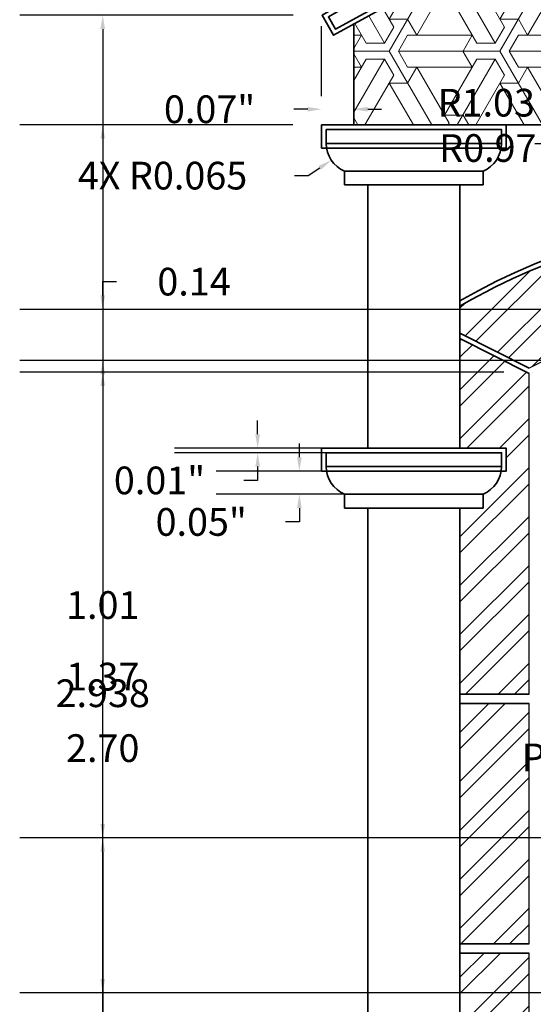
# Model space of a CAD drawing. Units: inches. Extents: x 19.36 to 24.97, y -1.46 to 4.09.
# Tile 2 of 4: x 19.36 to 20.47, y 0.85 to 2.98. Entities that reach past the tile are written whole.
import ezdxf

# ---------------------------------------------------------------- set-up
doc = ezdxf.new("R2010")
doc.units = ezdxf.units.IN
doc.header["$MEASUREMENT"] = 0
for name, color, linetype, lineweight in [('A-ANNO-DIMS', 2, 'Continuous', 18), ('A-COLS', 3, 'Continuous', 35), ('A-DOOR', 4, 'Continuous', 25), ('A-ELEV', 7, 'Continuous', 35), ('A-ELEV-PATT', 8, 'Continuous', 13)]:
    doc.layers.add(name, color=color, linetype=linetype, lineweight=lineweight)
doc.styles.get("Standard").update_dxf_attribs({"font": 'arial.ttf'})
doc.dimstyles.get("Standard").update_dxf_attribs({"dimtxt": 0.06, "dimasz": 0.03, "dimexe": 0.18, "dimexo": 0.0625, "dimgap": 0.09, "dimtad": 0, "dimtih": 1, "dimtoh": 1, "dimzin": 0, "dimdsep": 46, "dimlunit": 3, "dimtxsty": 'Standard', "dimcen": 0, "dimadec": 0, "dimazin": 0, "dimtfac": 1, "dimtofl": 0, "dimtmove": 0, "dimatfit": 3, "dimfxl": 1, "dimtolj": 1, "dimtzin": 0, "dimarcsym": 1})

# ---------------------------------------------------------------- blocks, each defined once
blk = doc.blocks.new('*D1')
at = {"layer": 'A-ANNO-DIMS', "color": 0, "lineweight": -2, "transparency": 16777216}
for p, q in [((19.8751, 2.08), (19.8751, 2.11)), ((20.0852, 2.05), (19.6951, 2.05)), ((20.0852, 2.04), (19.6951, 2.04)), ((19.8751, 2.01), (19.8751, 1.98)), ((19.8751, 1.98), (19.8451, 1.98))]:
    blk.add_line(p, q, dxfattribs=at)
at = {"layer": 'A-ANNO-DIMS', "color": 0, "transparency": 16777216}
for points in [[(19.8701, 2.08), (19.8801, 2.08), (19.8751, 2.05)], [(19.8701, 2.01), (19.8801, 2.01), (19.8751, 2.04)]]:
    blk.add_solid(points, dxfattribs=at)
at = {"layer": 'Defpoints', "color": 0, "transparency": 16777216}
for p in [(20.1477, 2.05), (19.8751, 2.04), (20.1477, 2.04)]:
    blk.add_point(p, dxfattribs=at)
at = {"layer": 'A-ANNO-DIMS', "color": 0, "transparency": 16777216, "insert": (19.6624, 1.98), "char_height": 0.06, "attachment_point": 5}
blk.add_mtext('\\A1;0.01"', dxfattribs=at)
blk = doc.blocks.new('*D2')
at = {"layer": 'A-ANNO-DIMS', "color": 0, "lineweight": -2, "transparency": 16777216}
for p, q in [((19.9655, 2.03), (19.9655, 2.06)), ((20.1117, 2), (19.7855, 2)), ((20.1117, 1.95), (19.7855, 1.95)), ((19.9655, 1.92), (19.9655, 1.89)), ((19.9655, 1.89), (19.9355, 1.89))]:
    blk.add_line(p, q, dxfattribs=at)
at = {"layer": 'A-ANNO-DIMS', "color": 0, "transparency": 16777216}
for points in [[(19.9605, 2.03), (19.9705, 2.03), (19.9655, 2)], [(19.9605, 1.92), (19.9705, 1.92), (19.9655, 1.95)]]:
    blk.add_solid(points, dxfattribs=at)
at = {"layer": 'Defpoints', "color": 0, "transparency": 16777216}
for p in [(20.1742, 2), (19.9655, 1.95), (20.1742, 1.95)]:
    blk.add_point(p, dxfattribs=at)
at = {"layer": 'A-ANNO-DIMS', "color": 0, "transparency": 16777216, "insert": (19.7528, 1.89), "char_height": 0.06, "attachment_point": 5}
blk.add_mtext('\\A1;0.05"', dxfattribs=at)
blk = doc.blocks.new('*D4')
at = {"layer": 'A-ANNO-DIMS', "color": 0, "lineweight": -2, "transparency": 16777216}
for p, q in [((20.0136, 2.8125), (20.0136, 2.9641)), ((20.0836, 2.8125), (20.0836, 2.9641)), ((19.9836, 2.7841), (19.9536, 2.7841)), ((20.1136, 2.7841), (20.1436, 2.7841))]:
    blk.add_line(p, q, dxfattribs=at)
at = {"layer": 'A-ANNO-DIMS', "color": 0, "transparency": 16777216}
for points in [[(19.9836, 2.7891), (19.9836, 2.7791), (20.0136, 2.7841)], [(20.1136, 2.7891), (20.1136, 2.7791), (20.0836, 2.7841)]]:
    blk.add_solid(points, dxfattribs=at)
at = {"layer": 'Defpoints', "color": 0, "transparency": 16777216}
for p in [(20.0136, 2.7841), (20.0136, 2.75), (20.0836, 2.75)]:
    blk.add_point(p, dxfattribs=at)
at = {"layer": 'A-ANNO-DIMS', "color": 0, "transparency": 16777216, "insert": (19.7709, 2.7841), "char_height": 0.06, "attachment_point": 5}
blk.add_mtext('\\A1;0.07"', dxfattribs=at)
blk = doc.blocks.new('PILASTER')
for p, q in [((20.1136, 2.65), (20.0636, 2.65)), ((20.1136, 2.65), (20.0636, 2.65)), ((20.0636, 2.65), (20.0636, 2.62)), ((20.1136, 2.65), (20.3136, 2.65)), ((20.1136, 2.65), (20.3136, 2.65)), ((20.3136, 2.65), (20.3636, 2.65)), ((20.3136, 2.65), (20.3636, 2.65)), ((20.3636, 2.62), (20.3636, 2.65)), ((20.1136, 2.62), (20.0636, 2.62)), ((20.1136, 2.62), (20.0636, 2.62)), ((20.1136, 2.05), (20.1136, 2.62)), ((20.1136, 2.62), (20.3136, 2.62)), ((20.1136, 2.62), (20.3136, 2.62)), ((20.3136, 2.05), (20.3136, 2.62)), ((20.3136, 2.62), (20.3636, 2.62)), ((20.3136, 2.62), (20.3636, 2.62)), ((20.1136, 1.95), (20.0636, 1.95)), ((20.0636, 1.95), (20.0636, 1.92)), ((20.1136, 1.95), (20.3136, 1.95)), ((20.3136, 1.95), (20.3636, 1.95)), ((20.3636, 1.92), (20.3636, 1.95)), ((20.1136, 1.92), (20.0636, 1.92)), ((20.1136, 0.15), (20.1136, 1.92)), ((20.1136, 1.92), (20.3136, 1.92)), ((20.3136, 0.15), (20.3136, 1.92)), ((20.3136, 1.92), (20.3636, 1.92))]:
    blk.add_line(p, q)
for centre, start, end in [((20.0886, 2.71), 180, 247.3801), ((20.3386, 2.71), 292.6199, 0), ((20.0886, 2.01), 180, 247.3801), ((20.3386, 2.01), 292.6199, 0)]:
    blk.add_arc(centre, 0.065, start, end)
blk = doc.blocks.new('*D17')
at = {"layer": 'A-ANNO-DIMS', "color": 0, "lineweight": -2, "transparency": 16777216}
for p, q in [((20.4761, 2.71), (20.9926, 2.71)), ((20.8126, 2.68), (20.8126, 1.501)), ((20.8126, 0.08), (20.8126, 1.259)), ((20.4761, 0.05), (20.9926, 0.05))]:
    blk.add_line(p, q, dxfattribs=at)
at = {"layer": 'A-ANNO-DIMS', "color": 0, "transparency": 16777216}
for points in [[(20.8076, 2.68), (20.8176, 2.68), (20.8126, 2.71)], [(20.8076, 0.08), (20.8176, 0.08), (20.8126, 0.05)]]:
    blk.add_solid(points, dxfattribs=at)
at = {"layer": 'Defpoints', "color": 0, "transparency": 16777216}
for p in [(20.4136, 2.71), (20.8126, 2.71), (20.4136, 0.05)]:
    blk.add_point(p, dxfattribs=at)
at = {"layer": 'A-ANNO-DIMS', "color": 0, "transparency": 16777216, "insert": (20.8126, 1.38), "char_height": 0.06, "attachment_point": 5}
blk.add_mtext('\\A1;PILASTER 2.66 TYP.', dxfattribs=at)
blk = doc.blocks.new('*D23')
at = {"layer": 'A-ANNO-DIMS', "color": 0, "lineweight": -2, "transparency": 16777216}
for p, q in [((20.9261, 1.2054), (19.3594, 1.2054)), ((19.5394, 1.1754), (19.5394, 0.7483)), ((19.5394, 0.08), (19.5394, 0.5071)), ((20.4111, 0.05), (19.3594, 0.05))]:
    blk.add_line(p, q, dxfattribs=at)
at = {"layer": 'A-ANNO-DIMS', "color": 0, "transparency": 16777216}
for points in [[(19.5344, 1.1754), (19.5444, 1.1754), (19.5394, 1.2054)], [(19.5344, 0.08), (19.5444, 0.08), (19.5394, 0.05)]]:
    blk.add_solid(points, dxfattribs=at)
at = {"layer": 'Defpoints', "color": 0, "transparency": 16777216}
for p in [(19.5394, 1.2054), (20.9886, 1.2054), (20.4736, 0.05)]:
    blk.add_point(p, dxfattribs=at)
at = {"layer": 'A-ANNO-DIMS', "color": 0, "transparency": 16777216, "insert": (19.5394, 0.6277), "char_height": 0.06, "attachment_point": 5}
blk.add_mtext('\\A1;1.16', dxfattribs=at)
blk = doc.blocks.new('*D24')
at = {"layer": 'A-ANNO-DIMS', "color": 0, "lineweight": -2, "transparency": 16777216}
for p, q in [((20.4089, 2.2147), (19.3594, 2.2147)), ((19.5394, 2.1847), (19.5394, 1.8307)), ((19.5394, 1.2354), (19.5394, 1.5894)), ((20.9261, 1.2054), (19.3594, 1.2054))]:
    blk.add_line(p, q, dxfattribs=at)
at = {"layer": 'A-ANNO-DIMS', "color": 0, "transparency": 16777216}
for points in [[(19.5344, 2.1847), (19.5444, 2.1847), (19.5394, 2.2147)], [(19.5344, 1.2354), (19.5444, 1.2354), (19.5394, 1.2054)]]:
    blk.add_solid(points, dxfattribs=at)
at = {"layer": 'Defpoints', "color": 0, "transparency": 16777216}
for p in [(19.5394, 2.2147), (20.4714, 2.2147), (20.9886, 1.2054)]:
    blk.add_point(p, dxfattribs=at)
at = {"layer": 'A-ANNO-DIMS', "color": 0, "transparency": 16777216, "insert": (19.5394, 1.71), "char_height": 0.06, "attachment_point": 5}
blk.add_mtext('\\A1;1.01', dxfattribs=at)
blk = doc.blocks.new('*D25')
at = {"layer": 'A-ANNO-DIMS', "color": 0, "lineweight": -2, "transparency": 16777216}
for p, q in [((19.5394, 2.3806), (19.5394, 2.4106)), ((19.5394, 2.4106), (19.5694, 2.4106)), ((20.9261, 2.3506), (19.3594, 2.3506)), ((20.4089, 2.2147), (19.3594, 2.2147)), ((19.5394, 2.1847), (19.5394, 2.1547))]:
    blk.add_line(p, q, dxfattribs=at)
at = {"layer": 'A-ANNO-DIMS', "color": 0, "transparency": 16777216}
for points in [[(19.5344, 2.3806), (19.5444, 2.3806), (19.5394, 2.3506)], [(19.5344, 2.1847), (19.5444, 2.1847), (19.5394, 2.2147)]]:
    blk.add_solid(points, dxfattribs=at)
at = {"layer": 'Defpoints', "color": 0, "transparency": 16777216}
for p in [(19.5394, 2.3506), (20.9886, 2.3506), (20.4714, 2.2147)]:
    blk.add_point(p, dxfattribs=at)
at = {"layer": 'A-ANNO-DIMS', "color": 0, "transparency": 16777216, "insert": (19.7372, 2.4106), "char_height": 0.06, "attachment_point": 5}
blk.add_mtext('\\A1;0.14', dxfattribs=at)
blk = doc.blocks.new('*D26')
at = {"layer": 'A-ANNO-DIMS', "color": 0, "lineweight": -2, "transparency": 16777216}
for p, q in [((19.9511, 2.75), (19.3594, 2.75)), ((19.5394, 2.72), (19.5394, 1.5206)), ((19.5394, 0.08), (19.5394, 1.2794)), ((19.9511, 0.05), (19.3594, 0.05))]:
    blk.add_line(p, q, dxfattribs=at)
at = {"layer": 'A-ANNO-DIMS', "color": 0, "transparency": 16777216}
for points in [[(19.5344, 2.72), (19.5444, 2.72), (19.5394, 2.75)], [(19.5344, 0.08), (19.5444, 0.08), (19.5394, 0.05)]]:
    blk.add_solid(points, dxfattribs=at)
at = {"layer": 'Defpoints', "color": 0, "transparency": 16777216}
for p in [(19.5394, 2.75), (20.0136, 2.75), (20.0136, 0.05)]:
    blk.add_point(p, dxfattribs=at)
at = {"layer": 'A-ANNO-DIMS', "color": 0, "transparency": 16777216, "insert": (19.5394, 1.4), "char_height": 0.06, "attachment_point": 5}
blk.add_mtext('\\A1;2.70', dxfattribs=at)
blk = doc.blocks.new('*D27')
at = {"layer": 'A-ANNO-DIMS', "color": 0, "lineweight": -2, "transparency": 16777216}
for p, q in [((19.9523, 2.9877), (19.3594, 2.9877)), ((19.5394, 2.9577), (19.5394, 1.6395)), ((19.5394, 0.08), (19.5394, 1.3982)), ((19.9511, 0.05), (19.3594, 0.05))]:
    blk.add_line(p, q, dxfattribs=at)
at = {"layer": 'A-ANNO-DIMS', "color": 0, "transparency": 16777216}
for points in [[(19.5344, 2.9577), (19.5444, 2.9577), (19.5394, 2.9877)], [(19.5344, 0.08), (19.5444, 0.08), (19.5394, 0.05)]]:
    blk.add_solid(points, dxfattribs=at)
at = {"layer": 'Defpoints', "color": 0, "transparency": 16777216}
for p in [(20.0148, 2.9877), (19.5394, 0.05), (20.0136, 0.05)]:
    blk.add_point(p, dxfattribs=at)
at = {"layer": 'A-ANNO-DIMS', "color": 0, "transparency": 16777216, "insert": (19.5394, 1.5189), "char_height": 0.06, "attachment_point": 5}
blk.add_mtext('\\A1;2.938', dxfattribs=at)
blk = doc.blocks.new('*D31')
at = {"layer": 'A-ANNO-DIMS', "color": 0, "lineweight": -2, "transparency": 16777216}
for p, q in [((20.9657, 2.2398), (19.3594, 2.2398)), ((19.5394, 2.2098), (19.5394, 1.6756)), ((19.5394, 0.9), (19.5394, 1.4342)), ((20.9661, 0.87), (19.3594, 0.87))]:
    blk.add_line(p, q, dxfattribs=at)
at = {"layer": 'A-ANNO-DIMS', "color": 0, "transparency": 16777216}
for points in [[(19.5344, 2.2098), (19.5444, 2.2098), (19.5394, 2.2398)], [(19.5344, 0.9), (19.5444, 0.9), (19.5394, 0.87)]]:
    blk.add_solid(points, dxfattribs=at)
at = {"layer": 'Defpoints', "color": 0, "transparency": 16777216}
for p in [(19.5394, 2.2398), (21.0282, 2.2398), (21.0286, 0.87)]:
    blk.add_point(p, dxfattribs=at)
at = {"layer": 'A-ANNO-DIMS', "color": 0, "transparency": 16777216, "insert": (19.5394, 1.5549), "char_height": 0.06, "attachment_point": 5}
blk.add_mtext('\\A1;1.37', dxfattribs=at)
blk = doc.blocks.new('*D39')
at = {"layer": 'A-ANNO-DIMS', "color": 0, "lineweight": -2, "transparency": 16777216}
for p, q in [((20.7496, 3.0257), (20.7796, 3.0257)), ((20.7796, 3.0257), (20.8546, 2.3729))]:
    blk.add_line(p, q, dxfattribs=at)
at = {"layer": 'A-ANNO-DIMS', "color": 0, "transparency": 16777216}
blk.add_solid([(20.8595, 2.3734), (20.8496, 2.3723), (20.858, 2.3431)], dxfattribs=at)
at = {"layer": 'Defpoints', "color": 0, "transparency": 16777216}
for p in [(20.858, 2.3431), (20.9886, 1.2054)]:
    blk.add_point(p, dxfattribs=at)
at = {"layer": 'A-ANNO-DIMS', "color": 0, "transparency": 16777216, "insert": (20.5527, 3.0257), "char_height": 0.06, "attachment_point": 5}
blk.add_mtext('\\A1;R1.15', dxfattribs=at)
blk = doc.blocks.new('*D44')
at = {"layer": 'A-ANNO-DIMS', "color": 0, "lineweight": -2, "transparency": 16777216}
for p, q in [((20.5672, 2.7983), (20.5972, 2.7983)), ((20.5972, 2.7983), (20.7369, 2.2301))]:
    blk.add_line(p, q, dxfattribs=at)
at = {"layer": 'A-ANNO-DIMS', "color": 0, "transparency": 16777216}
blk.add_solid([(20.7417, 2.2313), (20.732, 2.2289), (20.744, 2.2009)], dxfattribs=at)
at = {"layer": 'Defpoints', "color": 0, "transparency": 16777216}
for p in [(20.744, 2.2009), (20.9886, 1.2054)]:
    blk.add_point(p, dxfattribs=at)
at = {"layer": 'A-ANNO-DIMS', "color": 0, "transparency": 16777216, "insert": (20.3706, 2.7983), "char_height": 0.06, "attachment_point": 5}
blk.add_mtext('\\A1;R1.03', dxfattribs=at)
blk = doc.blocks.new('*D46')
at = {"layer": 'A-ANNO-DIMS', "color": 0, "lineweight": -2, "transparency": 16777216}
for p, q in [((20.5706, 2.7001), (20.6006, 2.7001)), ((20.6006, 2.7001), (20.7386, 2.1686))]:
    blk.add_line(p, q, dxfattribs=at)
at = {"layer": 'A-ANNO-DIMS', "color": 0, "transparency": 16777216}
blk.add_solid([(20.7434, 2.1699), (20.7337, 2.1674), (20.7461, 2.1396)], dxfattribs=at)
at = {"layer": 'Defpoints', "color": 0, "transparency": 16777216}
for p in [(20.7461, 2.1396), (20.9886, 1.2054)]:
    blk.add_point(p, dxfattribs=at)
at = {"layer": 'A-ANNO-DIMS', "color": 0, "transparency": 16777216, "insert": (20.374, 2.7001), "char_height": 0.06, "attachment_point": 5}
blk.add_mtext('\\A1;R0.97', dxfattribs=at)
blk = doc.blocks.new('*D47')
at = {"layer": 'A-ANNO-DIMS', "color": 0, "lineweight": -2, "transparency": 16777216}
for p, q in [((19.9849, 2.6403), (20.0098, 2.6571)), ((19.9549, 2.6403), (19.9849, 2.6403))]:
    blk.add_line(p, q, dxfattribs=at)
at = {"layer": 'A-ANNO-DIMS', "color": 0, "transparency": 16777216}
blk.add_solid([(20.007, 2.6612), (20.0125, 2.6529), (20.0347, 2.6738)], dxfattribs=at)
at = {"layer": 'Defpoints', "color": 0, "transparency": 16777216}
for p in [(20.0886, 2.71), (20.0347, 2.6738)]:
    blk.add_point(p, dxfattribs=at)
at = {"layer": 'A-ANNO-DIMS', "color": 0, "transparency": 16777216, "insert": (19.669, 2.6403), "char_height": 0.06, "attachment_point": 5}
blk.add_mtext('\\A1;4X R0.065', dxfattribs=at)

msp = doc.modelspace()

# ---------------------------------------------------------------- hatches: boundary and pattern name
at = {"layer": 'A-ELEV-PATT'}
h = msp.add_hatch(dxfattribs=at)
h.set_pattern_fill('ESCHER', color=256, scale=0.2)
h.paths.add_polyline_path([(20.9884, 3.4642), (20.0836, 2.9685), (20.0836, 2.75), (20.1136, 2.75), (20.3136, 2.75), (20.3636, 2.75), (20.4136, 2.75), (20.6081, 2.75, -0.635528), (21.3686, 2.75), (21.5636, 2.75), (21.6136, 2.75), (21.6636, 2.75), (21.8636, 2.75), (21.8936, 2.75), (21.8936, 2.9682)])
h = msp.add_hatch(dxfattribs=at)
h.set_pattern_fill('ANSI32', color=256, scale=0.2)
h.paths.add_polyline_path([(20.6294, 2.4913, 0.064491), (20.3136, 2.3574), (20.3136, 2.2989), (20.4636, 2.2231, -0.061889), (20.7287, 2.3207)])
h.paths.add_polyline_path([(20.9886, 2.5406, 0.066262), (20.6394, 2.4941), (20.7389, 2.323, -0.055018), (20.9886, 2.3506)])
h.paths.add_polyline_path([(21.3488, 2.491, 0.066519), (20.9986, 2.5405), (20.9986, 2.3505, -0.055118), (21.2486, 2.3207)])
h.paths.add_polyline_path([(21.6636, 2.3574, 0.062356), (21.3588, 2.4882), (21.2588, 2.3182, -0.0596), (21.5136, 2.2231), (21.6636, 2.2812)])
h.paths.add_polyline_path([(21.6636, 2.2704), (21.5136, 2.2124), (21.5136, 2.1846), (21.5136, 1.5166), (21.6636, 1.5166), (21.6636, 1.92), (21.6136, 1.92), (21.6136, 1.95, -0.261087), (21.5744, 2), (21.5636, 2), (21.5636, 2.05), (21.6136, 2.05), (21.6636, 2.05)])
h.paths.add_polyline_path([(21.6636, 1.4966), (21.5136, 1.4966), (21.5136, 0.9758), (21.6636, 0.9758)])
h.paths.add_polyline_path([(21.6636, 0.9558), (21.5136, 0.9558), (21.5136, 0.455), (21.6636, 0.455)])
h.paths.add_polyline_path([(21.6636, 0.435), (21.5136, 0.435), (21.5136, 0.08), (21.5636, 0.08), (21.5636, 0.1), (21.6136, 0.1), (21.6136, 0.15), (21.6636, 0.15)])
h.paths.add_polyline_path([(20.4636, 0.435), (20.3136, 0.435), (20.3136, 0.15), (20.3636, 0.15), (20.3636, 0.1), (20.4136, 0.1), (20.4136, 0.08), (20.4636, 0.08)])
h.paths.add_polyline_path([(20.4636, 0.9558), (20.3136, 0.9558), (20.3136, 0.455), (20.4636, 0.455)])
h.paths.add_polyline_path([(20.4636, 1.4966), (20.3136, 1.4966), (20.3136, 0.9758), (20.4636, 0.9758)])
h.paths.add_polyline_path([(20.4636, 2.1846), (20.4636, 2.2119), (20.3136, 2.2877), (20.3136, 2.05), (20.3636, 2.05), (20.4136, 2.05), (20.4136, 2), (20.4029, 2, -0.261087), (20.3636, 1.95), (20.3636, 1.92), (20.3136, 1.92), (20.3136, 1.5166), (20.4636, 1.5166)])

# ---------------------------------------------------------------- linework, layer by layer
at = {"layer": 'A-DOOR'}
for p, q in [((20.4636, 2.1846), (20.4636, 2.2119)), ((20.4714, 2.2147), (20.4714, 2.2147))]:
    msp.add_line(p, q, dxfattribs=at)
for points in [[(20.4636, 1.5166), (20.4636, 2.1846)], [(20.4636, 0.9758), (20.4636, 1.4966)], [(20.4636, 0.455), (20.4636, 0.9558)]]:
    msp.add_lwpolyline(points, dxfattribs=at)
msp.add_arc((20.9886, 1.2054), 1.1452, 76.8803, 117.2863, dxfattribs=at)
at = {"layer": 'A-ELEV'}
for p, q in [((20.0836, 2.75), (20.0836, 2.9685)), ((20.0136, 2.75), (20.0836, 2.75)), ((20.4636, 2.2231), (20.3136, 2.2989)), ((20.4636, 2.2119), (20.3136, 2.2877)), ((20.3136, 1.5166), (20.4636, 1.5166)), ((20.4636, 1.5166), (20.3136, 1.5166)), ((20.3136, 1.4966), (20.4636, 1.4966)), ((20.4636, 1.4966), (20.3136, 1.4966)), ((20.4636, 0.9758), (20.3136, 0.9758)), ((20.3136, 0.9758), (20.4636, 0.9758)), ((20.4636, 0.9558), (20.3136, 0.9558)), ((20.3136, 0.9558), (20.4636, 0.9558))]:
    msp.add_line(p, q, dxfattribs=at)
for points in [[(21.937, 2.9444), (21.962, 2.9877), (20.9884, 3.5451), (20.0148, 2.9877), (20.0398, 2.9444), (20.9884, 3.4642)], [(21.9332, 2.9579), (21.9483, 2.9841), (20.9884, 3.5336), (20.0285, 2.9841), (20.0436, 2.9579), (20.9884, 3.4756)], [(20.0136, 2.75), (20.0636, 2.75), (20.1136, 2.75), (20.3136, 2.75), (20.3636, 2.75), (20.4136, 2.75), (20.4136, 2.7), (20.3636, 2.7), (20.3136, 2.7), (20.1136, 2.7), (20.0636, 2.7), (20.0136, 2.7)], [(20.0236, 2.74), (20.0636, 2.74), (20.1136, 2.74), (20.3136, 2.74), (20.3636, 2.74), (20.4036, 2.74), (20.4036, 2.71), (20.3636, 2.71), (20.3136, 2.71), (20.1136, 2.71), (20.0636, 2.71), (20.0236, 2.71)], [(20.0136, 2.05), (20.0636, 2.05), (20.1136, 2.05), (20.3136, 2.05), (20.3636, 2.05), (20.4136, 2.05), (20.4136, 2), (20.3636, 2), (20.3136, 2), (20.1136, 2), (20.0636, 2), (20.0136, 2)], [(20.0236, 2.04), (20.0636, 2.04), (20.1136, 2.04), (20.3136, 2.04), (20.3636, 2.04), (20.4036, 2.04), (20.4036, 2.01), (20.3636, 2.01), (20.3136, 2.01), (20.1136, 2.01), (20.0636, 2.01), (20.0236, 2.01)]]:
    msp.add_lwpolyline(points, close=True, dxfattribs=at)
for points in [[(20.0136, 2.75), (20.0636, 2.75)], [(20.4136, 2.75), (20.6081, 2.75)]]:
    msp.add_lwpolyline(points, dxfattribs=at)
for radius, start, end in [(1.3452, 59.8817, 120.1183), (1.3352, 105.6078, 120.3675)]:
    msp.add_arc((20.9886, 1.2054), radius, start, end, dxfattribs=at)

# ---------------------------------------------------------------- block references
at = {"layer": 'A-COLS'}
msp.add_blockref('PILASTER', (0, 0), dxfattribs=at)

# ---------------------------------------------------------------- dimensions: what is measured, and where the dimension line sits
at = {"layer": 'A-ANNO-DIMS'}
for mpoint, picture, middle in [((20.858, 2.3431), '*D39', (20.5527, 3.0257)), ((20.744, 2.2009), '*D44', (20.3706, 2.7983)), ((20.7461, 2.1396), '*D46', (20.374, 2.7001))]:
    dim = msp.add_radius_dim(center=(20.9886, 1.2054), mpoint=mpoint, dimstyle='Standard', override={"dimdec": 2, "dimlfac": 1, "dimrnd": 0, "dimzin": 0, "dimdsep": 46, "dimlunit": 2}, dxfattribs=at)
    dim.commit()
    dim.dimension.update_dxf_attribs({"geometry": picture, "text_midpoint": middle, "dimtype": 164})
for base, p1, p2, override, picture, middle in [((19.5394, 0.05), (20.0148, 2.9877), (20.0136, 0.05), {"dimdec": 3, "dimlfac": 1, "dimrnd": 0, "dimzin": 0, "dimdsep": 46, "dimlunit": 2}, '*D27', (19.5394, 1.5189)), ((19.5394, 2.75), (20.0136, 0.05), (20.0136, 2.75), {"dimdec": 2, "dimlfac": 1, "dimrnd": 0, "dimzin": 0, "dimdsep": 46, "dimlunit": 2}, '*D26', (19.5394, 1.4)), ((19.5394, 2.3506), (20.4714, 2.2147), (20.9886, 2.3506), {"dimdec": 2, "dimlfac": 1, "dimrnd": 0, "dimzin": 0, "dimdsep": 46, "dimlunit": 2}, '*D25', (19.7372, 2.4106)), ((19.5394, 2.2398), (21.0286, 0.87), (21.0282, 2.2398), {"dimdec": 2, "dimlfac": 1, "dimrnd": 0, "dimzin": 0, "dimdsep": 46, "dimlunit": 2}, '*D31', (19.5394, 1.5549)), ((19.5394, 2.2147), (20.9886, 1.2054), (20.4714, 2.2147), {"dimdec": 2, "dimlfac": 1, "dimrnd": 0, "dimzin": 0, "dimdsep": 46, "dimlunit": 2}, '*D24', (19.5394, 1.71)), ((19.8751, 2.04), (20.1477, 2.05), (20.1477, 2.04), {"dimclrd": 0, "dimclre": 0, "dimclrt": 0}, '*D1', (19.6624, 1.98)), ((19.9655, 1.95), (20.1742, 2), (20.1742, 1.95), {"dimclrd": 0, "dimclre": 0, "dimclrt": 0}, '*D2', (19.7528, 1.89)), ((19.5394, 1.2054), (20.4736, 0.05), (20.9886, 1.2054), {"dimdec": 2, "dimlfac": 1, "dimrnd": 0, "dimzin": 0, "dimdsep": 46, "dimlunit": 2}, '*D23', (19.5394, 0.6277))]:
    dim = msp.add_linear_dim(base=base, p1=p1, p2=p2, angle=90, dimstyle='Standard', override=override, dxfattribs=at)
    dim.commit()
    dim.dimension.update_dxf_attribs({"geometry": picture, "text_midpoint": middle})
dim = msp.add_linear_dim(base=(20.0136, 2.7841), p1=(20.0836, 2.75), p2=(20.0136, 2.75), dimstyle='Standard', override={"dimclrd": 0, "dimclre": 0, "dimclrt": 0}, dxfattribs=at)
dim.commit()
dim.dimension.update_dxf_attribs({"geometry": '*D4', "text_midpoint": (19.7709, 2.7841)})
dim = msp.add_radius_dim(center=(20.0886, 2.71), mpoint=(20.0347, 2.6738), text='4X <>', dimstyle='Standard', override={"dimdec": 3, "dimlfac": 1, "dimrnd": 0, "dimzin": 0, "dimdsep": 46, "dimlunit": 2}, dxfattribs=at)
dim.commit()
dim.dimension.update_dxf_attribs({"geometry": '*D47', "text_midpoint": (19.669, 2.6403)})
dim = msp.add_linear_dim(base=(20.8126, 2.71), p1=(20.4136, 0.05), p2=(20.4136, 2.71), angle=90, text='PILASTER <> TYP.', dimstyle='Standard', override={"dimdec": 2, "dimrnd": 0, "dimzin": 0, "dimlunit": 2}, dxfattribs=at)
dim.commit()
dim.dimension.update_dxf_attribs({"geometry": '*D17', "text_midpoint": (20.8126, 1.38)})

doc.saveas('drawing.dxf')
